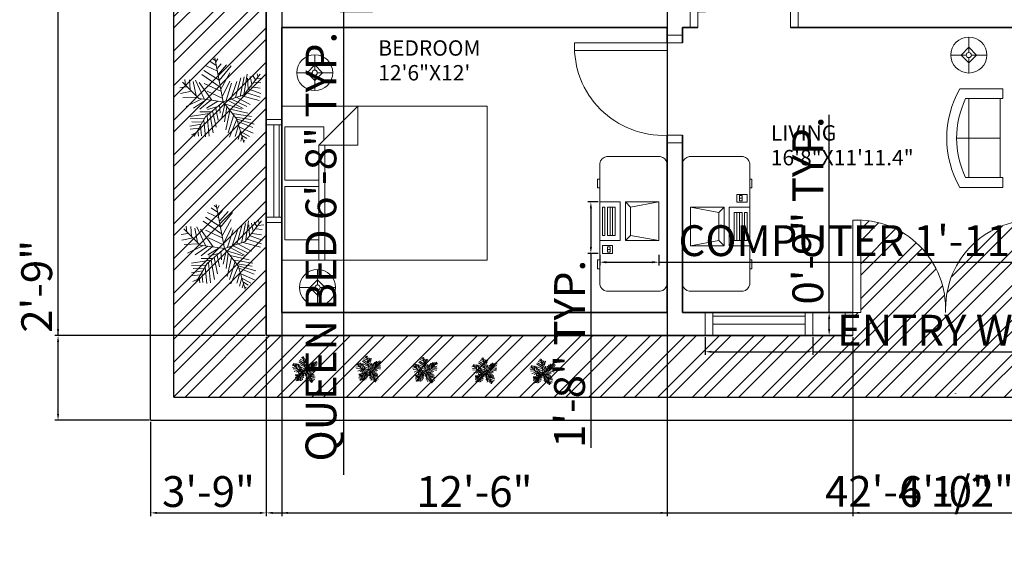
# Model space of a CAD drawing. Units: inches. Extents: x 2297 to 3143, y 440 to 1351.
# Tile 1 of 6: x 2342 to 2725, y 501 to 704. Entities that reach past the tile are written whole.
import ezdxf

# ---------------------------------------------------------------- set-up
doc = ezdxf.new("R2010")
doc.units = ezdxf.units.IN
for name, color, linetype, lineweight in [('A-ANNO-DIMS', 2, 'Continuous', 18), ('A-AREA-IDEN', 7, 'Continuous', 18), ('A-DOOR', 4, 'Continuous', 20), ('A-EQPM', 8, 'Continuous', 18), ('A-FURN', 8, 'Continuous', 18), ('A-GLAZ', 4, 'Continuous', 18), ('A-WALL', 7, 'Continuous', 35), ('C-PROP', 7, 'Continuous', 25), ('C-SITE-PATT', 252, 'Continuous', 13), ('E-LITE', 9, 'Continuous', 13), ('L-PLNT', 3, 'Continuous', 13)]:
    doc.layers.add(name, color=color, linetype=linetype, lineweight=lineweight)
doc.styles.get("Standard").update_dxf_attribs({"font": 'arial.ttf'})
doc.dimstyles.new('ISO-25', dxfattribs={"dimtxt": 12, "dimasz": 2.5, "dimexe": 1.25, "dimexo": 0.625, "dimtad": 1, "dimdec": 1, "dimlunit": 3, "dimtxsty": 'Standard', "dimcen": 2.5, "dimadec": 0, "dimazin": 0, "dimtfac": 1, "dimtdec": 1, "dimtmove": 0, "dimatfit": 3, "dimfxl": 1, "dimarcsym": 0})

# ---------------------------------------------------------------- blocks, each defined once
blk = doc.blocks.new('Bed - Queen')
for p, q in [((0, -80.00003), (0, 0)), ((0, 0), (59.99999, 0)), ((59.99999, 0), (59.99999, -80.00003)), ((7.99999, -1.2), (28.79998, -1.2)), ((7.99999, -14.4), (7.99999, -1.2)), ((28.79998, -1.2), (28.79998, -14.4)), ((31.19999, -1.2), (51.99999, -1.2)), ((31.19999, -14.4), (31.19999, -1.2)), ((51.99999, -1.2), (51.99999, -16.4)), ((0, -14.4), (44.8, -14.4)), ((59.99999, -29.6), (44.8, -14.4)), ((44.8, -14.4), (44.8, -29.6)), ((44.8, -16.8), (0, -16.8)), ((51.99999, -16.4), (46.79936, -16.4)), ((44.8, -29.6), (59.99999, -29.6)), ((59.99999, -80.00003), (0, -80.00003))]:
    blk.add_line(p, q)
blk = doc.blocks.new('Sofa - Roundback Loveseat 5 ft.')
for p, q in [((-24, -33.99998), (-24, -11.46958)), ((0, -32.44198), (0, -5.99998)), ((24.00004, -33.99998), (24.00004, -11.46958)), ((-23.9998, -13.38178), (23.99986, -13.38178)), ((-24, -32.44198), (24.00004, -32.44198))]:
    blk.add_line(p, q)
for points in [[(-24, -33.99998), (-30, -33.99998), (-30, -7.99998)], [(30.00004, -7.99998), (30.00004, -33.99998), (24.00004, -33.99998)]]:
    blk.add_lwpolyline(points)
for centre, radius, start, end in [((0, -60.24998), 60.24998, 60.13715, 119.8628), ((0, -61.38438), 55.38444, 64.32083, 115.6792)]:
    blk.add_arc(centre, radius, start, end)
blk = doc.blocks.new('*U16')
for p, q in [((-8.737, 47.138), (-17.069, 52.711)), ((-10.186, 53.64), (-13.084, 55.962)), ((0, 0), (-10.5, 57)), ((-9.099, 51.782), (-6.563, 55.962)), ((-5.114, 28.097), (-24.676, 40.636)), ((-7.288, 39.707), (-21.778, 46.673)), ((-7.65, 43.423), (-2.578, 49.46)), ((-5.839, 35.992), (4.667, 48.067)), ((-5.114, 27.632), (10.463, 46.673)), ((-48.585, 21.131), (-49.309, 29.026)), ((-43.513, 28.561), (-42.427, 15.558)), ((-38.442, 26.239), (-34.819, 7.663)), ((-35.544, 28.097), (-24.314, 3.947)), ((-3.665, 19.273), (-27.574, 35.527)), ((-2.941, 16.486), (8.652, 37.85)), ((-1.129, 6.734), (9.014, 26.704)), ((10.101, 3.483), (17.708, 26.239)), ((16.259, 5.805), (23.142, 31.348)), ((22.055, 7.198), (27.489, 32.277)), ((27, 9), (48, 36)), ((27.127, 9.056), (31.112, 35.992)), ((31.836, 30.883), (32.561, 16.486)), ((35.096, 32.741), (37.27, 22.524)), ((38.719, 34.134), (41.979, 28.561)), ((40.53, 25.775), (48.862, 24.846)), ((43.791, 29.954), (51.036, 30.883)), ((44.153, 36.456), (45.239, 32.741)), ((-47.498, 19.737), (-55.83, 18.344)), ((-40.615, 13.7), (-55.105, 10.913)), ((-31.5, 4.5), (-52.5, 25.5)), ((-14.533, 2.09), (-30.834, 25.31)), ((-24.314, 23.917), (-2.941, 13.7)), ((-20.691, 13.7), (-1.129, 4.876)), ((3.942, 1.625), (11.187, 24.381)), ((33.285, 16.486), (48.862, 10.913)), ((36.183, 19.737), (48.137, 17.88)), ((-33.37, 6.269), (-52.207, 5.34)), ((-28.299, 3.483), (-47.86, -5.805)), ((-21.416, 3.018), (-38.079, -8.128)), ((0, 0), (-31.5, 4.5)), ((-15.982, 2.09), (-30.11, -9.521)), ((0, 0), (-22.5, -19.5)), ((-6.563, 1.161), (-21.416, -8.128)), ((0, 0), (27, 9)), ((0, 0), (18, -22.5)), ((6.478, 1.625), (26.04, -8.592)), ((11.187, 3.483), (30.749, -5.805)), ((18.07, 5.805), (35.096, -3.483)), ((24.229, 7.663), (46.688, 1.625)), ((29.662, 12.307), (48.137, 6.269)), ((-6.563, -5.805), (-19.967, -9.985)), ((-13.446, -11.378), (-8.737, -32.741)), ((-9.461, -8.592), (-6.201, -23.453)), ((-4.752, -3.483), (-3.665, -14.629)), ((2.493, -3.019), (-1.491, -20.202)), ((1.769, -2.555), (24.229, -9.521)), ((5.029, -6.27), (2.131, -25.775)), ((9.014, -11.378), (3.58, -35.992)), ((7.565, -9.056), (32.198, -14.629)), ((-17.431, -15.094), (-42.789, -18.809)), ((-24.314, -21.596), (-42.427, -22.06)), ((-22.5, -19.5), (-37.5, -45)), ((-15.257, -12.772), (-30.11, -12.772)), ((-25.038, -23.918), (-22.865, -45.281)), ((-20.691, -18.345), (-17.793, -44.352)), ((-17.069, -15.094), (-12.721, -40.172)), ((14.085, -16.951), (6.478, -40.172)), ((18.07, -22.524), (8.289, -45.745)), ((12.274, -15.094), (36.907, -18.809)), ((16.259, -19.738), (36.183, -22.989)), ((18, -22.5), (27, -52.5)), ((18.433, -22.524), (40.53, -29.026)), ((19.157, -25.311), (38.719, -33.206)), ((-28.299, -29.026), (-42.789, -31.348)), ((-30.834, -34.135), (-42.427, -35.528)), ((-26.849, -26.24), (-40.253, -25.775)), ((-32.646, -36.921), (-31.921, -44.352)), ((-29.023, -30.884), (-27.936, -43.887)), ((20.244, -30.419), (15.897, -44.816)), ((22.78, -37.85), (19.519, -48.532)), ((21.331, -32.741), (39.081, -40.636)), ((-34.457, -39.708), (-40.978, -42.494)), ((22.78, -38.314), (34.372, -44.816)), ((24.591, -45.745), (23.142, -50.854)), ((24.591, -43.423), (30.749, -47.603)), ((26.764, -49.925), (28.213, -50.854))]:
    blk.add_line(p, q)
blk = doc.blocks.new('Lamp - Table')
for p, q in [((0, 7), (0, 1)), ((-1, 0), (-7, 0)), ((0, 3), (-3, 0)), ((-3, 0), (0, -3)), ((3, 0), (0, 3)), ((0, -3), (3, 0)), ((1, 0), (7, 0)), ((0, -1), (0, -7))]:
    blk.add_line(p, q)
for radius in [7, 1]:
    blk.add_circle((0, 0), radius)
blk = doc.blocks.new('Desk - 30 x 60 in.')
for p, q in [((-26.999995, 0), (26.999995, 0)), ((-29.999995, -27), (-29.999995, -3)), ((29.999995, -3), (29.999995, -27)), ((26.999995, -30), (-26.999995, -30)), ((-20.000005, -30), (-20.000005, -31)), ((-16.000005, -31), (-16.000005, -30)), ((15.999995, -31), (15.999995, -30)), ((19.999995, -30), (19.999995, -31)), ((-20.000005, -31), (-16.000005, -31)), ((19.999995, -31), (15.999995, -31))]:
    blk.add_line(p, q)
for centre, start, end in [((-26.499995, -3.5), 98.1301, 171.8699), ((26.499995, -3.5), 8.130102, 81.8699), ((-26.499995, -26.5), 188.1301, 261.8699), ((26.499995, -26.5), 278.1301, 351.8699)]:
    blk.add_arc(centre, 3.535534, start, end)
blk = doc.blocks.new('Computer Terminal')
for p, q in [((-10, 11.5), (5, 11.5)), ((-8, 0.5), (-10, 11.5)), ((-10, -1.5), (-10, 11.5)), ((5, 11.5), (3, 0.5)), ((5, 11.5), (5, -1.5)), ((-10, -1.5), (-8, 0.5)), ((3, 0.5), (-8, 0.5)), ((3, 0.5), (5, -1.5)), ((5, -1.5), (-10, -1.5)), ((-10, -11.5), (-10, -3.5)), ((-10, -3.5), (5, -3.5)), ((5, -3.5), (5, -11.5)), ((-8, -5.5), (-8, -8.5)), ((3, -5.5), (-8, -5.5)), ((3, -6.5), (-8, -6.5)), ((-8, -7.5), (3, -7.5)), ((3, -8.5), (3, -5.5)), ((10, -6.5), (7, -6.5)), ((7, -6.5), (7, -10.5)), ((9.5, -7.5), (7.5, -7.5)), ((7.5, -7.5), (7.5, -8.5)), ((8.5, -7.5), (8.5, -8.5)), ((9.5, -8.5), (9.5, -7.5)), ((10, -10.5), (10, -6.5)), ((-8, -8.5), (3, -8.5)), ((-8, -9.5), (-8, -10.5)), ((3, -9.5), (-8, -9.5)), ((-8, -10.5), (3, -10.5)), ((3, -10.5), (3, -9.5)), ((7, -10.5), (10, -10.5)), ((7.5, -8.5), (9.5, -8.5)), ((5, -11.5), (-10, -11.5))]:
    blk.add_line(p, q)
blk = doc.blocks.new('DOOR-36IN-6IN-JAMB')
for p, q in [((0, 6), (0, 0)), ((3, 6), (3, 0)), ((39, 6), (39, 0)), ((42, 6), (42, 0))]:
    blk.add_line(p, q)
blk.add_lwpolyline([(39, 6), (36, 6), (36, 42), (39, 42)], close=True)
blk.add_arc((37.5, 7.5), 34.53, 87.5104, 182.4896)
blk = doc.blocks.new('WIN-36IN-6IN-WALL')
for p, q in [((6, 40), (0, 40)), ((6, 38), (0, 38)), ((3, 38), (3, 2)), ((5, 38), (5, 2)), ((0, 2), (6, 2)), ((0, 0), (6, 0))]:
    blk.add_line(p, q)
blk = doc.blocks.new('WIN-36IN-9IN-WALL')
for p, q in [((0, 9), (0, 0)), ((3, 9), (3, 0)), ((39, 0), (39, 9)), ((42, 0), (42, 9)), ((3, 7.5), (39, 7.5)), ((3, 4.5), (39, 4.5))]:
    blk.add_line(p, q)
blk = doc.blocks.new('*D35')
at = {"layer": 'A-ANNO-DIMS', "color": 0, "lineweight": -2, "transparency": 16777216}
for p, q in [((2568, 612.02), (2568, 607.95)), ((2591, 612.02), (2591, 607.95)), ((2570.5, 609.2), (2588.5, 609.2)), ((2591, 609.2), (2777.67, 609.2))]:
    blk.add_line(p, q, dxfattribs=at)
at = {"layer": 'A-ANNO-DIMS', "color": 0, "transparency": 16777216}
for points in [[(2570.5, 609.61), (2570.5, 608.78), (2568, 609.2)], [(2588.5, 609.61), (2588.5, 608.78), (2591, 609.2)]]:
    blk.add_solid(points, dxfattribs=at)
at = {"layer": 'Defpoints', "color": 0, "transparency": 16777216}
for p in [(2568, 612.65), (2591, 612.65), (2591, 609.2)]:
    blk.add_point(p, dxfattribs=at)
at = {"layer": 'A-ANNO-DIMS', "color": 0, "transparency": 16777216, "insert": (2685.59, 616.03), "char_height": 12, "attachment_point": 5}
blk.add_mtext('COMPUTER 1\'-11" TYP.', dxfattribs=at)
blk = doc.blocks.new('*D36')
at = {"layer": 'A-ANNO-DIMS', "color": 0, "lineweight": -2, "transparency": 16777216}
for p, q in [((2567.38, 632.65), (2563.3, 632.65)), ((2564.55, 630.15), (2564.55, 615.15)), ((2567.38, 612.65), (2563.3, 612.65)), ((2564.55, 612.65), (2564.55, 536.88))]:
    blk.add_line(p, q, dxfattribs=at)
at = {"layer": 'A-ANNO-DIMS', "color": 0, "transparency": 16777216}
for points in [[(2564.14, 630.15), (2564.97, 630.15), (2564.55, 632.65)], [(2564.14, 615.15), (2564.97, 615.15), (2564.55, 612.65)]]:
    blk.add_solid(points, dxfattribs=at)
at = {"layer": 'Defpoints', "color": 0, "transparency": 16777216}
for p in [(2568, 632.65), (2564.55, 612.65), (2568, 612.65)]:
    blk.add_point(p, dxfattribs=at)
at = {"layer": 'A-ANNO-DIMS', "color": 0, "transparency": 16777216, "insert": (2557.8, 573.51), "char_height": 12, "attachment_point": 5, "rotation": 90}
blk.add_mtext('1\'-8" TYP.', dxfattribs=at)
blk = doc.blocks.new('*D37')
at = {"layer": 'A-ANNO-DIMS', "color": 0, "lineweight": -2, "transparency": 16777216}
for p, q in [((2479.6, 786.63), (2466.97, 786.63)), ((2468.22, 784.13), (2468.22, 709.13)), ((2479.6, 706.63), (2466.97, 706.63)), ((2468.22, 706.63), (2468.22, 526.36))]:
    blk.add_line(p, q, dxfattribs=at)
at = {"layer": 'A-ANNO-DIMS', "color": 0, "transparency": 16777216}
for points in [[(2467.8, 784.13), (2468.64, 784.13), (2468.22, 786.63)], [(2467.8, 709.13), (2468.64, 709.13), (2468.22, 706.63)]]:
    blk.add_solid(points, dxfattribs=at)
at = {"layer": 'Defpoints', "color": 0, "transparency": 16777216}
for p in [(2480.22, 786.63), (2468.22, 706.63), (2480.22, 706.63)]:
    blk.add_point(p, dxfattribs=at)
at = {"layer": 'A-ANNO-DIMS', "color": 0, "transparency": 16777216, "insert": (2461.02, 615.25), "char_height": 12, "attachment_point": 5, "rotation": 90}
blk.add_mtext('QUEEN BED 6\'-8" TYP.', dxfattribs=at)
blk = doc.blocks.new('*D59')
at = {"layer": 'A-ANNO-DIMS', "color": 0, "lineweight": -2, "transparency": 16777216}
for p, q in [((2608.99, 580.01), (2608.99, 573.08)), ((2650.99, 580.01), (2650.99, 573.08)), ((2611.49, 574.33), (2648.49, 574.33)), ((2650.99, 574.33), (2866.94, 574.33))]:
    blk.add_line(p, q, dxfattribs=at)
at = {"layer": 'A-ANNO-DIMS', "color": 0, "transparency": 16777216}
for points in [[(2611.49, 574.75), (2611.49, 573.92), (2608.99, 574.33)], [(2648.49, 574.75), (2648.49, 573.92), (2650.99, 574.33)]]:
    blk.add_solid(points, dxfattribs=at)
at = {"layer": 'Defpoints', "color": 0, "transparency": 16777216}
for p in [(2608.99, 580.63), (2650.99, 580.63), (2650.99, 574.33)]:
    blk.add_point(p, dxfattribs=at)
at = {"layer": 'A-ANNO-DIMS', "color": 0, "transparency": 16777216, "insert": (2760.21, 581.17), "char_height": 12, "attachment_point": 5}
blk.add_mtext('ENTRY WINDOW 3\'-6" TYP.', dxfattribs=at)
blk = doc.blocks.new('*D60')
at = {"layer": 'A-ANNO-DIMS', "color": 0, "lineweight": -2, "transparency": 16777216}
for p, q in [((2657.29, 589.63), (2657.29, 666.53)), ((2651.61, 589.63), (2658.54, 589.63)), ((2657.29, 583.13), (2657.29, 587.13)), ((2651.61, 580.63), (2658.54, 580.63))]:
    blk.add_line(p, q, dxfattribs=at)
at = {"layer": 'A-ANNO-DIMS', "color": 0, "transparency": 16777216}
for points in [[(2656.87, 587.13), (2657.7, 587.13), (2657.29, 589.63)], [(2656.87, 583.13), (2657.7, 583.13), (2657.29, 580.63)]]:
    blk.add_solid(points, dxfattribs=at)
at = {"layer": 'Defpoints', "color": 0, "transparency": 16777216}
for p in [(2650.99, 589.63), (2657.29, 589.63), (2650.99, 580.63)]:
    blk.add_point(p, dxfattribs=at)
at = {"layer": 'A-ANNO-DIMS', "color": 0, "transparency": 16777216, "insert": (2650.54, 629.33), "char_height": 12, "attachment_point": 5, "rotation": 90}
blk.add_mtext('0\'-9" TYP.', dxfattribs=at)
blk = doc.blocks.new('*D69')
at = {"layer": 'A-ANNO-DIMS', "color": 0, "lineweight": -2, "transparency": 16777216}
for p, q in [((2946.69, 700.01), (2946.69, 510.33)), ((2438.19, 580.01), (2438.19, 510.33)), ((2440.69, 511.58), (2944.19, 511.58))]:
    blk.add_line(p, q, dxfattribs=at)
at = {"layer": 'A-ANNO-DIMS', "color": 0, "transparency": 16777216}
for points in [[(2440.69, 512), (2440.69, 511.17), (2438.19, 511.58)], [(2944.19, 512), (2944.19, 511.17), (2946.69, 511.58)]]:
    blk.add_solid(points, dxfattribs=at)
at = {"layer": 'Defpoints', "color": 0, "transparency": 16777216}
for p in [(2946.69, 700.63), (2438.19, 580.63), (2946.69, 511.58)]:
    blk.add_point(p, dxfattribs=at)
at = {"layer": 'A-ANNO-DIMS', "color": 0, "transparency": 16777216, "insert": (2692.44, 518.41), "char_height": 12, "attachment_point": 5}
blk.add_mtext('42\'-4 1/2"', dxfattribs=at)
blk = doc.blocks.new('*D70')
at = {"layer": 'A-ANNO-DIMS', "color": 0, "lineweight": -2, "transparency": 16777216}
for p, q in [((2392.57, 1207.63), (2355.89, 1207.63)), ((2357.14, 583.13), (2357.14, 1205.13)), ((2437.57, 580.63), (2355.89, 580.63))]:
    blk.add_line(p, q, dxfattribs=at)
at = {"layer": 'A-ANNO-DIMS', "color": 0, "transparency": 16777216}
for points in [[(2356.73, 1205.13), (2357.56, 1205.13), (2357.14, 1207.63)], [(2356.73, 583.13), (2357.56, 583.13), (2357.14, 580.63)]]:
    blk.add_solid(points, dxfattribs=at)
at = {"layer": 'Defpoints', "color": 0, "transparency": 16777216}
for p in [(2357.14, 1207.63), (2393.19, 1207.63), (2438.19, 580.63)]:
    blk.add_point(p, dxfattribs=at)
at = {"layer": 'A-ANNO-DIMS', "color": 0, "transparency": 16777216, "insert": (2350.39, 894.13), "char_height": 12, "attachment_point": 5, "rotation": 90}
blk.add_mtext('52\'-3"', dxfattribs=at)
blk = doc.blocks.new('*D71')
at = {"layer": 'A-ANNO-DIMS', "color": 0, "lineweight": -2, "transparency": 16777216}
for p, q in [((2438.19, 580.01), (2438.19, 510.33)), ((2393.19, 547.01), (2393.19, 510.33)), ((2395.69, 511.58), (2435.69, 511.58))]:
    blk.add_line(p, q, dxfattribs=at)
at = {"layer": 'A-ANNO-DIMS', "color": 0, "transparency": 16777216}
for points in [[(2395.69, 512), (2395.69, 511.17), (2393.19, 511.58)], [(2435.69, 512), (2435.69, 511.17), (2438.19, 511.58)]]:
    blk.add_solid(points, dxfattribs=at)
at = {"layer": 'Defpoints', "color": 0, "transparency": 16777216}
for p in [(2438.19, 580.63), (2393.19, 547.63), (2438.19, 511.58)]:
    blk.add_point(p, dxfattribs=at)
at = {"layer": 'A-ANNO-DIMS', "color": 0, "transparency": 16777216, "insert": (2415.69, 518.34), "char_height": 12, "attachment_point": 5}
blk.add_mtext('3\'-9"', dxfattribs=at)
blk = doc.blocks.new('*D73')
at = {"layer": 'A-ANNO-DIMS', "color": 0, "lineweight": -2, "transparency": 16777216}
for p, q in [((2357.14, 580.63), (2357.14, 616.49)), ((2437.57, 580.63), (2355.89, 580.63)), ((2357.14, 550.13), (2357.14, 578.13)), ((2392.57, 547.63), (2355.89, 547.63))]:
    blk.add_line(p, q, dxfattribs=at)
at = {"layer": 'A-ANNO-DIMS', "color": 0, "transparency": 16777216}
for points in [[(2356.73, 578.13), (2357.56, 578.13), (2357.14, 580.63)], [(2356.73, 550.13), (2357.56, 550.13), (2357.14, 547.63)]]:
    blk.add_solid(points, dxfattribs=at)
at = {"layer": 'Defpoints', "color": 0, "transparency": 16777216}
for p in [(2357.14, 580.63), (2438.19, 580.63), (2393.19, 547.63)]:
    blk.add_point(p, dxfattribs=at)
at = {"layer": 'A-ANNO-DIMS', "color": 0, "transparency": 16777216, "insert": (2350.39, 599.81), "char_height": 12, "attachment_point": 5, "rotation": 90}
blk.add_mtext('2\'-9"', dxfattribs=at)
blk = doc.blocks.new('*D77')
at = {"layer": 'A-ANNO-DIMS', "color": 0, "lineweight": -2, "transparency": 16777216}
for p, q in [((2444.19, 874.01), (2444.19, 510.33)), ((2594.19, 874.01), (2594.19, 510.33)), ((2446.69, 511.58), (2591.69, 511.58))]:
    blk.add_line(p, q, dxfattribs=at)
at = {"layer": 'A-ANNO-DIMS', "color": 0, "transparency": 16777216}
for points in [[(2446.69, 512), (2446.69, 511.17), (2444.19, 511.58)], [(2591.69, 512), (2591.69, 511.17), (2594.19, 511.58)]]:
    blk.add_solid(points, dxfattribs=at)
at = {"layer": 'Defpoints', "color": 0, "transparency": 16777216}
for p in [(2444.19, 874.63), (2594.19, 874.63), (2594.19, 511.58)]:
    blk.add_point(p, dxfattribs=at)
at = {"layer": 'A-ANNO-DIMS', "color": 0, "transparency": 16777216, "insert": (2519.19, 518.34), "char_height": 12, "attachment_point": 5}
blk.add_mtext('12\'-6"', dxfattribs=at)
blk = doc.blocks.new('*D81')
at = {"layer": 'A-ANNO-DIMS', "color": 0, "lineweight": -2, "transparency": 16777216}
for p, q in [((2666.57, 580.01), (2666.57, 510.33)), ((2738.57, 580.01), (2738.57, 510.33)), ((2669.07, 511.58), (2736.07, 511.58))]:
    blk.add_line(p, q, dxfattribs=at)
at = {"layer": 'A-ANNO-DIMS', "color": 0, "transparency": 16777216}
for points in [[(2669.07, 512), (2669.07, 511.17), (2666.57, 511.58)], [(2736.07, 512), (2736.07, 511.17), (2738.57, 511.58)]]:
    blk.add_solid(points, dxfattribs=at)
at = {"layer": 'Defpoints', "color": 0, "transparency": 16777216}
for p in [(2666.57, 580.63), (2738.57, 580.63), (2738.57, 511.58)]:
    blk.add_point(p, dxfattribs=at)
at = {"layer": 'A-ANNO-DIMS', "color": 0, "transparency": 16777216, "insert": (2702.57, 518.34), "char_height": 12, "attachment_point": 5}
blk.add_mtext('6\'-0"', dxfattribs=at)

msp = doc.modelspace()

# ---------------------------------------------------------------- hatches: boundary and pattern name
at = {"layer": 'C-SITE-PATT'}
h = msp.add_hatch(dxfattribs=at)
h.set_pattern_fill('ANSI32', color=256)
h.paths.add_polyline_path([(2438.19, 1198.63), (2402.19, 1198.63), (2402.19, 556.63), (2667.43, 556.63), (2742.43, 556.63), (2946.69, 556.63), (2982.69, 556.63), (2982.69, 1117.63), (2982.69, 1123.63), (2982.69, 1198.63), (2946.69, 1198.63), (2946.69, 1117.63), (2946.69, 700.63), (2806.19, 700.63), (2806.19, 580.63), (2738.57, 580.63), (2738.57, 589.63), (2735.57, 589.63), (2735.57, 625.63, 0.402069), (2702.6, 591.13, 0.401544), (2669.57, 625.63), (2669.57, 589.63), (2666.57, 589.63), (2666.57, 580.63), (2438.19, 580.63)])
h.paths.add_polyline_path([(2706.46, 558.2, -0.000472), (2706.46, 558.13, -0.000473)], flags=16)
h.paths.add_polyline_path([(2875.15, 576.11), (2920.92, 576.11), (2920.92, 585.31), (2875.15, 585.31)], flags=24)
h.paths.add_polyline_path([(2875.13, 585.74), (2915.96, 585.74), (2915.96, 595.05), (2875.13, 595.05)], flags=24)
h.paths.add_polyline_path([(2646.52, 1069.72), (2687.63, 1069.72), (2687.63, 1078.92), (2646.52, 1078.92)], flags=25)
h.paths.add_polyline_path([(2646.5, 1079.35), (2686.39, 1079.35), (2686.39, 1088.65), (2646.5, 1088.65)], flags=25)

# ---------------------------------------------------------------- linework, layer by layer
at = {"layer": 'A-DOOR'}
for p, q in [((2663.57, 589.63), (2663.57, 580.63)), ((2666.57, 589.63), (2666.57, 580.63))]:
    msp.add_line(p, q, dxfattribs=at)
msp.add_lwpolyline([(2666.57, 589.63), (2669.57, 589.63), (2669.57, 625.63), (2666.57, 625.63)], close=True, dxfattribs=at)
for centre, radius, start, end in [((2668.07, 591.13), 34.53, 357.5104, 92.4896), ((2737.07, 591.2), 34.47, 87.5057, 180.1084)]:
    msp.add_arc(centre, radius, start, end, dxfattribs=at)
at = {"layer": 'A-WALL'}
for p, q in [((2438.19, 580.63), (2438.19, 1198.63)), ((2444.19, 589.63), (2444.19, 700.63)), ((2444.19, 700.63), (2594.19, 700.63)), ((2594.19, 694.63), (2594.19, 700.63)), ((2600.19, 700.63), (2606.19, 700.63)), ((2600.19, 694.63), (2600.19, 700.63)), ((2642.19, 700.63), (2800.19, 700.63)), ((2594.19, 589.63), (2594.19, 658.63)), ((2600.19, 589.63), (2600.19, 658.63)), ((2444.19, 589.63), (2594.19, 589.63)), ((2600.19, 589.63), (2666.57, 589.63)), ((2438.19, 580.63), (2666.57, 580.63))]:
    msp.add_line(p, q, dxfattribs=at)
at = {"layer": 'C-PROP'}
for p, q in [((2393.19, 547.63), (2393.19, 1207.63)), ((2402.19, 556.63), (2402.19, 1198.63)), ((2402.19, 556.63), (2667.43, 556.63)), ((2444.19, 556.63), (2667.43, 556.63)), ((2600.19, 556.63), (2742.43, 556.63))]:
    msp.add_line(p, q, dxfattribs=at)
msp.add_lwpolyline([(2393.19, 547.63), (2742.43, 547.63)], dxfattribs=at)
for centre, radius, start, end in [((2671.93, 558.13), 34.53, 0, 0.1083), ((2740.93, 558.2), 34.47, 179.9999, 180.1084)]:
    msp.add_arc(centre, radius, start, end, dxfattribs=at)

# ---------------------------------------------------------------- block references
at = {"layer": 'A-DOOR', "extrusion": (0, 0, -1), "zscale": -1}
msp.add_blockref('DOOR-36IN-6IN-JAMB', (-2645.19, 700.63), dxfattribs=at)
at = {"layer": 'A-DOOR', "rotation": 89.99999999999928}
msp.add_blockref('DOOR-36IN-6IN-JAMB', (2600.19, 655.63), dxfattribs=at)
at = {"layer": 'A-EQPM'}
for p, rotation in [((2579.5, 622.65), 270), ((2614.88, 625.62), 89.99999999999999)]:
    msp.add_blockref('Computer Terminal', p, dxfattribs=dict(at, rotation=rotation))
at = {"layer": 'A-FURN'}
for name, p, xscale, yscale, zscale, rotation in [('Sofa - Roundback Loveseat 5 ft.', (2703.05, 657.51), 0.6411223808005011, 0.6411223808005011, 0.6411223808005011, 89.99999999999999), ('Desk - 30 x 60 in.', (2594.19, 624.13), 0.8729228900222988, 0.8729228900222988, 0.8729228900222988, 270), ('Desk - 30 x 60 in.', (2600.19, 624.13), 0.8729228900222988, 0.8729228900222988, 0.8729228900222988, 89.99999999999999)]:
    msp.add_blockref(name, p, dxfattribs=dict(at, xscale=xscale, yscale=yscale, zscale=zscale, rotation=rotation))
at = {"layer": 'A-FURN', "rotation": 90}
msp.add_blockref('Bed - Queen', (2444.19, 609.93), dxfattribs=at)
at = {"layer": 'A-GLAZ'}
for name, p in [('WIN-36IN-6IN-WALL', (2438.19, 624.71)), ('WIN-36IN-9IN-WALL', (2608.99, 580.63))]:
    msp.add_blockref(name, p, dxfattribs=at)
at = {"layer": 'E-LITE'}
for p in [(2711.65, 689.87), (2457.05, 683), (2458.15, 599.35)]:
    msp.add_blockref('Lamp - Table', p, dxfattribs=at)
at = {"layer": 'L-PLNT'}
for p, xscale, yscale, zscale in [((2421.35, 671.62), 0.3005060358918508, 0.3005060358918508, 0.3005060358918508), ((2421.89, 614.51), 0.3005060358918508, 0.3005060358918508, 0.3005060358918508), ((2453.44, 567.15), 0.0926114314353741, 0.0926114314353741, 0.0926114314353741), ((2478.21, 567.37), 0.0926114314353741, 0.0926114314353741, 0.0926114314353741), ((2500.15, 566.94), 0.0926114314353741, 0.0926114314353741, 0.0926114314353741), ((2523.4, 566.72), 0.0926114314353741, 0.0926114314353741, 0.0926114314353741), ((2545.99, 566.29), 0.0926114314353741, 0.0926114314353741, 0.0926114314353741)]:
    msp.add_blockref('*U16', p, dxfattribs=dict(at, xscale=xscale, yscale=yscale, zscale=zscale))

# ---------------------------------------------------------------- texts
at = {"layer": 'A-AREA-IDEN'}
for s, p in [('BEDROOM', (2481.77, 689.61)), ('12\'6"X12\'', (2481.77, 679.97)), ('LIVING', (2634.57, 656.56)), ('16\'8"X11\'11.4"', (2634.57, 646.92))]:
    msp.add_text(s, height=6, dxfattribs=at).set_placement(p)

# ---------------------------------------------------------------- dimensions: what is measured, and where the dimension line sits
at = {"layer": 'A-ANNO-DIMS'}
for base, p1, p2, picture, middle in [((2357.14, 1207.63), (2438.19, 580.63), (2393.19, 1207.63), '*D70', (2350.39, 894.13)), ((2357.14, 580.63), (2393.19, 547.63), (2438.19, 580.63), '*D73', (2350.39, 599.81))]:
    dim = msp.add_linear_dim(base=base, p1=p1, p2=p2, angle=90, dimstyle='ISO-25', override={"dimdec": 1, "dimlfac": 1, "dimrnd": 0, "dimzin": 1, "dimdsep": 46, "dimlunit": 4, "dimfrac": 2}, dxfattribs=at)
    dim.commit()
    dim.dimension.update_dxf_attribs({"geometry": picture, "text_midpoint": middle})
for base, p1, p2, picture, middle in [((2594.19, 511.58), (2444.19, 874.63), (2594.19, 874.63), '*D77', (2519.19, 518.34)), ((2946.69, 511.58), (2438.19, 580.63), (2946.69, 700.63), '*D69', (2692.44, 518.41)), ((2438.19, 511.58), (2393.19, 547.63), (2438.19, 580.63), '*D71', (2415.69, 518.34)), ((2738.57, 511.58), (2666.57, 580.63), (2738.57, 580.63), '*D81', (2702.57, 518.34))]:
    dim = msp.add_linear_dim(base=base, p1=p1, p2=p2, dimstyle='ISO-25', override={"dimdec": 1, "dimlfac": 1, "dimrnd": 0, "dimzin": 1, "dimdsep": 46, "dimlunit": 4, "dimfrac": 2}, dxfattribs=at)
    dim.commit()
    dim.dimension.update_dxf_attribs({"geometry": picture, "text_midpoint": middle})
for base, p1, p2, angle, text, picture, middle in [((2468.22, 706.63), (2480.22, 786.63), (2480.22, 706.63), 270, 'QUEEN BED <> TYP.', '*D37', (2461.02, 615.25)), ((2657.29, 589.63), (2650.99, 580.63), (2650.99, 589.63), 90, '<> TYP.', '*D60', (2650.54, 629.33)), ((2564.55, 612.65), (2568, 632.65), (2568, 612.65), 270, '<> TYP.', '*D36', (2557.8, 573.51))]:
    dim = msp.add_linear_dim(base=base, p1=p1, p2=p2, angle=angle, text=text, dimstyle='ISO-25', override={"dimdec": 1, "dimlfac": 1, "dimrnd": 0, "dimzin": 1, "dimdsep": 46, "dimlunit": 4, "dimfrac": 2}, dxfattribs=at)
    dim.commit()
    dim.dimension.update_dxf_attribs({"geometry": picture, "text_midpoint": middle})
for base, p1, p2, text, picture, middle in [((2591, 609.2), (2568, 612.65), (2591, 612.65), 'COMPUTER <> TYP.', '*D35', (2685.59, 616.03)), ((2650.99, 574.33), (2608.99, 580.63), (2650.99, 580.63), 'ENTRY WINDOW <> TYP.', '*D59', (2760.21, 581.17))]:
    dim = msp.add_linear_dim(base=base, p1=p1, p2=p2, text=text, dimstyle='ISO-25', override={"dimdec": 1, "dimlfac": 1, "dimrnd": 0, "dimzin": 1, "dimdsep": 46, "dimlunit": 4, "dimfrac": 2}, dxfattribs=at)
    dim.commit()
    dim.dimension.update_dxf_attribs({"geometry": picture, "text_midpoint": middle})

doc.saveas('drawing.dxf')
